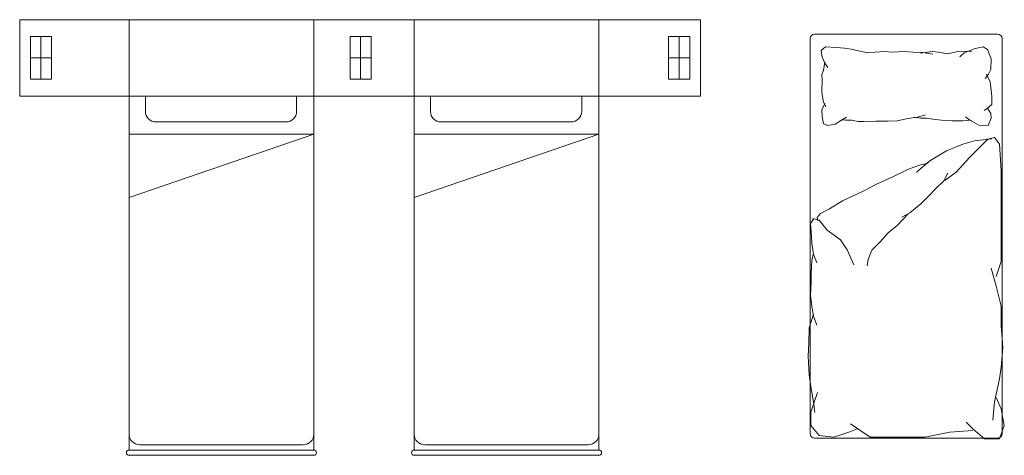
# Model space of a CAD drawing. Units: inches. Extents: x 1994 to 3075, y 3517 to 3950.
# Tile 1 of 58: x 1993.6955 to 1993.8965, y 3553.2238 to 3553.3128. Entities that reach past the tile are written whole.
import ezdxf

# ---------------------------------------------------------------- set-up
doc = ezdxf.new("R2010")
doc.units = ezdxf.units.IN
doc.layers.add('A-FURN-REFR', color=8, linetype='Continuous', lineweight=13)

msp = doc.modelspace()

# ---------------------------------------------------------------- linework, layer by layer
at = {"layer": 'A-FURN-REFR'}
for p, q in [((1993.83446, 3553.31278), (1993.69555, 3553.31278)), ((1993.69555, 3553.29715), (1993.69555, 3553.31278)), ((1993.71786, 3553.29715), (1993.71786, 3553.31278)), ((1993.75557, 3553.29715), (1993.75557, 3553.31278)), ((1993.77603, 3553.29715), (1993.77603, 3553.31278)), ((1993.81374, 3553.29715), (1993.81374, 3553.31278)), ((1993.83446, 3553.29715), (1993.83446, 3553.31278)), ((1993.70206, 3553.30931), (1993.69772, 3553.30931)), ((1993.69772, 3553.30063), (1993.69772, 3553.30931)), ((1993.69989, 3553.30063), (1993.69989, 3553.30931)), ((1993.70206, 3553.30063), (1993.70206, 3553.30931)), ((1993.76295, 3553.30063), (1993.76295, 3553.30931)), ((1993.76729, 3553.30931), (1993.76295, 3553.30931)), ((1993.76512, 3553.30063), (1993.76512, 3553.30931)), ((1993.76729, 3553.30063), (1993.76729, 3553.30931)), ((1993.83229, 3553.30931), (1993.82795, 3553.30931)), ((1993.82795, 3553.30063), (1993.82795, 3553.30931)), ((1993.83012, 3553.30063), (1993.83012, 3553.30931)), ((1993.83229, 3553.30063), (1993.83229, 3553.30931)), ((1993.85775, 3553.30985), (1993.89507, 3553.30985)), ((1993.85683, 3553.22822), (1993.85683, 3553.30893)), ((1993.85999, 3553.30722), (1993.8591, 3553.30651)), ((1993.86219, 3553.30713), (1993.85999, 3553.30722)), ((1993.86387, 3553.30696), (1993.86219, 3553.30713)), ((1993.89217, 3553.30722), (1993.89049, 3553.30687)), ((1993.89305, 3553.30669), (1993.89217, 3553.30722)), ((1993.89599, 3553.30893), (1993.89599, 3553.22822)), ((1993.8591, 3553.30651), (1993.85928, 3553.3051)), ((1993.85928, 3553.3051), (1993.85981, 3553.30387)), ((1993.86519, 3553.30678), (1993.86387, 3553.30696)), ((1993.86669, 3553.30643), (1993.86519, 3553.30678)), ((1993.86863, 3553.30599), (1993.86669, 3553.30643)), ((1993.87004, 3553.30616), (1993.86836, 3553.30599)), ((1993.87206, 3553.30625), (1993.87004, 3553.30616)), ((1993.87356, 3553.30616), (1993.87206, 3553.30625)), ((1993.87603, 3553.30625), (1993.87356, 3553.30616)), ((1993.87788, 3553.30616), (1993.87603, 3553.30625)), ((1993.87982, 3553.30607), (1993.87788, 3553.30616)), ((1993.88176, 3553.30625), (1993.87934, 3553.30592)), ((1993.88185, 3553.30572), (1993.87982, 3553.30607)), ((1993.883, 3553.30616), (1993.88176, 3553.30625)), ((1993.88485, 3553.30581), (1993.883, 3553.30616)), ((1993.88696, 3553.30625), (1993.88485, 3553.30581)), ((1993.88829, 3553.30634), (1993.88696, 3553.30625)), ((1993.88829, 3553.30599), (1993.88741, 3553.30519)), ((1993.89049, 3553.30687), (1993.88829, 3553.30599)), ((1993.88983, 3553.30628), (1993.88829, 3553.30634)), ((1993.89375, 3553.30475), (1993.89305, 3553.30669)), ((1993.70206, 3553.30497), (1993.69772, 3553.30497)), ((1993.76729, 3553.30497), (1993.76295, 3553.30497)), ((1993.83229, 3553.30497), (1993.82795, 3553.30497)), ((1993.85981, 3553.30414), (1993.85955, 3553.30237)), ((1993.85981, 3553.30387), (1993.86043, 3553.30299)), ((1993.89367, 3553.30263), (1993.89375, 3553.30475)), ((1993.85955, 3553.30237), (1993.85919, 3553.30157)), ((1993.85919, 3553.30157), (1993.85928, 3553.30025)), ((1993.89252, 3553.30078), (1993.89322, 3553.30166)), ((1993.89281, 3553.30165), (1993.89358, 3553.30007)), ((1993.89322, 3553.30166), (1993.89367, 3553.30263)), ((1993.70206, 3553.30063), (1993.69772, 3553.30063)), ((1993.76729, 3553.30063), (1993.76295, 3553.30063)), ((1993.83229, 3553.30063), (1993.82795, 3553.30063)), ((1993.85928, 3553.30025), (1993.85919, 3553.29831)), ((1993.89358, 3553.30007), (1993.89367, 3553.29893)), ((1993.83446, 3553.29715), (1993.69555, 3553.29715)), ((1993.71786, 3553.22813), (1993.71786, 3553.29715)), ((1993.7212, 3553.29405), (1993.7212, 3553.29715)), ((1993.75205, 3553.29405), (1993.75205, 3553.29715)), ((1993.75557, 3553.22487), (1993.75557, 3553.29715)), ((1993.77603, 3553.22813), (1993.77603, 3553.29715)), ((1993.77937, 3553.29405), (1993.77937, 3553.29715)), ((1993.81022, 3553.29405), (1993.81022, 3553.29715)), ((1993.81374, 3553.22487), (1993.81374, 3553.29715)), ((1993.85919, 3553.29831), (1993.85928, 3553.29734)), ((1993.85928, 3553.29734), (1993.85955, 3553.29601)), ((1993.89367, 3553.29893), (1993.89393, 3553.29707)), ((1993.89393, 3553.29707), (1993.89393, 3553.29548)), ((1993.85981, 3553.29568), (1993.85919, 3553.29434)), ((1993.85955, 3553.29601), (1993.86007, 3553.29495)), ((1993.89393, 3553.29548), (1993.89305, 3553.29469)), ((1993.85919, 3553.29434), (1993.85928, 3553.29301)), ((1993.88035, 3553.29337), (1993.87877, 3553.29284)), ((1993.89305, 3553.29469), (1993.89234, 3553.29425)), ((1993.89305, 3553.29469), (1993.89367, 3553.29363)), ((1993.89367, 3553.29363), (1993.89375, 3553.29266)), ((1993.74988, 3553.29188), (1993.72337, 3553.29188)), ((1993.80805, 3553.29188), (1993.78154, 3553.29188)), ((1993.85928, 3553.29301), (1993.85955, 3553.29151)), ((1993.85955, 3553.29151), (1993.86043, 3553.29116)), ((1993.86043, 3553.29116), (1993.86193, 3553.29143)), ((1993.86193, 3553.29143), (1993.86325, 3553.29222)), ((1993.86413, 3553.29222), (1993.86318, 3553.29231)), ((1993.86325, 3553.29222), (1993.86422, 3553.29284)), ((1993.86536, 3553.29222), (1993.86413, 3553.29222)), ((1993.8666, 3553.29195), (1993.86536, 3553.29222)), ((1993.86783, 3553.29195), (1993.8666, 3553.29195)), ((1993.87021, 3553.29204), (1993.86783, 3553.29195)), ((1993.87277, 3553.29204), (1993.87021, 3553.29204)), ((1993.87462, 3553.29213), (1993.87277, 3553.29204)), ((1993.87674, 3553.29257), (1993.87462, 3553.29213)), ((1993.87877, 3553.29284), (1993.87674, 3553.29257)), ((1993.87938, 3553.29266), (1993.87806, 3553.29284)), ((1993.88062, 3553.29266), (1993.87938, 3553.29266)), ((1993.88185, 3553.29248), (1993.88062, 3553.29266)), ((1993.88361, 3553.29222), (1993.88185, 3553.29248)), ((1993.88573, 3553.29213), (1993.88361, 3553.29222)), ((1993.88802, 3553.29213), (1993.88573, 3553.29213)), ((1993.88979, 3553.29222), (1993.88802, 3553.29213)), ((1993.88935, 3553.29231), (1993.88855, 3553.29293)), ((1993.89128, 3553.29125), (1993.88935, 3553.29231)), ((1993.89314, 3553.29116), (1993.89128, 3553.29125)), ((1993.89375, 3553.29266), (1993.89314, 3553.29116)), ((1993.75557, 3553.28937), (1993.71786, 3553.28937)), ((1993.75557, 3553.28937), (1993.71786, 3553.27644)), ((1993.81374, 3553.28937), (1993.77603, 3553.28937)), ((1993.81374, 3553.28937), (1993.77603, 3553.27644)), ((1993.88801, 3553.28735), (1993.88464, 3553.286)), ((1993.89038, 3553.28802), (1993.88801, 3553.28735)), ((1993.89394, 3553.28842), (1993.89038, 3553.28802)), ((1993.89308, 3553.28836), (1993.89139, 3553.28667)), ((1993.89443, 3553.2887), (1993.89308, 3553.28836)), ((1993.89544, 3553.28735), (1993.89443, 3553.2887)), ((1993.89578, 3553.28195), (1993.89544, 3553.28735)), ((1993.88464, 3553.286), (1993.88126, 3553.28397)), ((1993.89139, 3553.28667), (1993.88936, 3553.28465)), ((1993.87918, 3553.28306), (1993.87693, 3553.28221)), ((1993.88126, 3553.28397), (1993.87856, 3553.28161)), ((1993.88089, 3553.28349), (1993.87918, 3553.28306)), ((1993.88936, 3553.28465), (1993.88666, 3553.28161)), ((1993.87693, 3553.28221), (1993.87372, 3553.28071)), ((1993.88496, 3553.28146), (1993.88411, 3553.27985)), ((1993.88666, 3553.28161), (1993.8843, 3553.27992)), ((1993.89578, 3553.27621), (1993.89578, 3553.28195)), ((1993.8704, 3553.27921), (1993.86751, 3553.27771)), ((1993.87372, 3553.28071), (1993.8704, 3553.27921)), ((1993.88411, 3553.27985), (1993.88239, 3553.27824)), ((1993.86751, 3553.27771), (1993.86344, 3553.27578)), ((1993.88239, 3553.27824), (1993.88111, 3553.27685)), ((1993.86344, 3553.27578), (1993.86076, 3553.27417)), ((1993.8794, 3553.27514), (1993.87715, 3553.27332)), ((1993.88111, 3553.27685), (1993.8794, 3553.27514)), ((1993.89578, 3553.26946), (1993.89578, 3553.27621)), ((1993.85894, 3553.27321), (1993.8583, 3553.27235)), ((1993.86076, 3553.27417), (1993.85894, 3553.27321)), ((1993.87683, 3553.2731), (1993.87458, 3553.27075)), ((1993.87715, 3553.27332), (1993.87554, 3553.27246)), ((1993.85755, 3553.27205), (1993.85692, 3553.27116)), ((1993.85692, 3553.27116), (1993.85704, 3553.26952)), ((1993.85865, 3553.27182), (1993.8573, 3553.27216)), ((1993.8583, 3553.27235), (1993.85841, 3553.27171)), ((1993.86034, 3553.2698), (1993.85865, 3553.27182)), ((1993.85704, 3553.26952), (1993.85717, 3553.26713)), ((1993.86304, 3553.26778), (1993.86034, 3553.2698)), ((1993.87276, 3553.26925), (1993.87115, 3553.26743)), ((1993.87458, 3553.27075), (1993.87276, 3553.26925)), ((1993.89578, 3553.26339), (1993.89578, 3553.26946)), ((1993.85717, 3553.26713), (1993.85755, 3553.26486)), ((1993.86439, 3553.26575), (1993.86304, 3553.26778)), ((1993.87115, 3553.26743), (1993.86944, 3553.26571)), ((1993.85755, 3553.26511), (1993.85717, 3553.2636)), ((1993.86574, 3553.26271), (1993.86439, 3553.26575)), ((1993.86944, 3553.26571), (1993.86869, 3553.26378)), ((1993.85717, 3553.2636), (1993.85704, 3553.26095)), ((1993.85755, 3553.26486), (1993.85818, 3553.26309)), ((1993.86869, 3553.26378), (1993.86847, 3553.2625)), ((1993.89477, 3553.26035), (1993.89578, 3553.26339)), ((1993.85704, 3553.26095), (1993.85704, 3553.25918)), ((1993.89477, 3553.25833), (1993.89375, 3553.26204)), ((1993.85704, 3553.25918), (1993.85692, 3553.2564)), ((1993.89578, 3553.25428), (1993.89477, 3553.25833)), ((1993.85692, 3553.2564), (1993.85717, 3553.25426)), ((1993.85717, 3553.25426), (1993.85755, 3553.25224)), ((1993.89578, 3553.25023), (1993.89578, 3553.25428)), ((1993.85666, 3553.24985), (1993.85755, 3553.25262)), ((1993.85755, 3553.25224), (1993.85818, 3553.25035)), ((1993.85654, 3553.24669), (1993.85666, 3553.24985)), ((1993.89612, 3553.24584), (1993.89578, 3553.25023)), ((1993.85641, 3553.24404), (1993.85654, 3553.24669)), ((1993.89578, 3553.24179), (1993.89612, 3553.24584)), ((1993.85666, 3553.24026), (1993.85641, 3553.24404)), ((1993.89544, 3553.23943), (1993.89578, 3553.24179)), ((1993.85704, 3553.23736), (1993.85666, 3553.24026)), ((1993.89443, 3553.23471), (1993.89544, 3553.23943)), ((1993.85755, 3553.23471), (1993.85704, 3553.23736)), ((1993.85764, 3553.23462), (1993.85831, 3553.23664)), ((1993.89477, 3553.23563), (1993.89578, 3553.23327)), ((1993.85696, 3553.23259), (1993.85764, 3553.23462)), ((1993.8578, 3553.23256), (1993.85755, 3553.23471)), ((1993.89409, 3553.231), (1993.89443, 3553.23471)), ((1993.89578, 3553.23327), (1993.89645, 3553.22989)), ((1993.85696, 3553.22989), (1993.85696, 3553.23259)), ((1993.85865, 3553.22787), (1993.85696, 3553.22989)), ((1993.86641, 3553.22922), (1993.86472, 3553.22854)), ((1993.86911, 3553.22753), (1993.86506, 3553.23023)), ((1993.89004, 3553.22888), (1993.88531, 3553.22854)), ((1993.89004, 3553.22922), (1993.88869, 3553.23057)), ((1993.8924, 3553.22719), (1993.89004, 3553.22922)), ((1993.89645, 3553.22989), (1993.89544, 3553.22719)), ((1993.71786, 3553.22813), (1993.71786, 3553.22487)), ((1993.77603, 3553.22813), (1993.77603, 3553.22487)), ((1993.89507, 3553.2273), (1993.85775, 3553.2273)), ((1993.86169, 3553.22753), (1993.85865, 3553.22787)), ((1993.86472, 3553.22854), (1993.86169, 3553.22753)), ((1993.87316, 3553.22753), (1993.86911, 3553.22753)), ((1993.88025, 3553.22753), (1993.87316, 3553.22753)), ((1993.88531, 3553.22854), (1993.88025, 3553.22753)), ((1993.89544, 3553.22719), (1993.8924, 3553.22719)), ((1993.75557, 3553.22487), (1993.71786, 3553.22487)), ((1993.7534, 3553.22596), (1993.72003, 3553.22596)), ((1993.81374, 3553.22487), (1993.77603, 3553.22487)), ((1993.81157, 3553.22596), (1993.7782, 3553.22596)), ((1993.75557, 3553.22379), (1993.71786, 3553.22379)), ((1993.81374, 3553.22379), (1993.77603, 3553.22379))]:
    msp.add_line(p, q, dxfattribs=at)
for centre, radius, start, end in [((1993.85775, 3553.30893), 0.000921, 90, 180), ((1993.89507, 3553.30893), 0.000921, 0, 90), ((1993.72337, 3553.29405), 0.00217, 180, 270), ((1993.74988, 3553.29405), 0.00217, 270, 0), ((1993.78154, 3553.29405), 0.00217, 180, 270), ((1993.80805, 3553.29405), 0.00217, 270, 0), ((1993.72003, 3553.22813), 0.00217, 180, 270), ((1993.7534, 3553.22813), 0.00217, 270, 0), ((1993.7782, 3553.22813), 0.00217, 180, 270), ((1993.81157, 3553.22813), 0.00217, 270, 0), ((1993.85775, 3553.22822), 0.000921, 180, 270), ((1993.89507, 3553.22822), 0.000921, 270, 0), ((1993.71786, 3553.22433), 0.000543, 90, 270), ((1993.75557, 3553.22433), 0.000543, 270, 90), ((1993.77603, 3553.22433), 0.000543, 90, 270), ((1993.81374, 3553.22433), 0.000543, 270, 90)]:
    msp.add_arc(centre, radius, start, end, dxfattribs=at)

doc.saveas('drawing.dxf')
